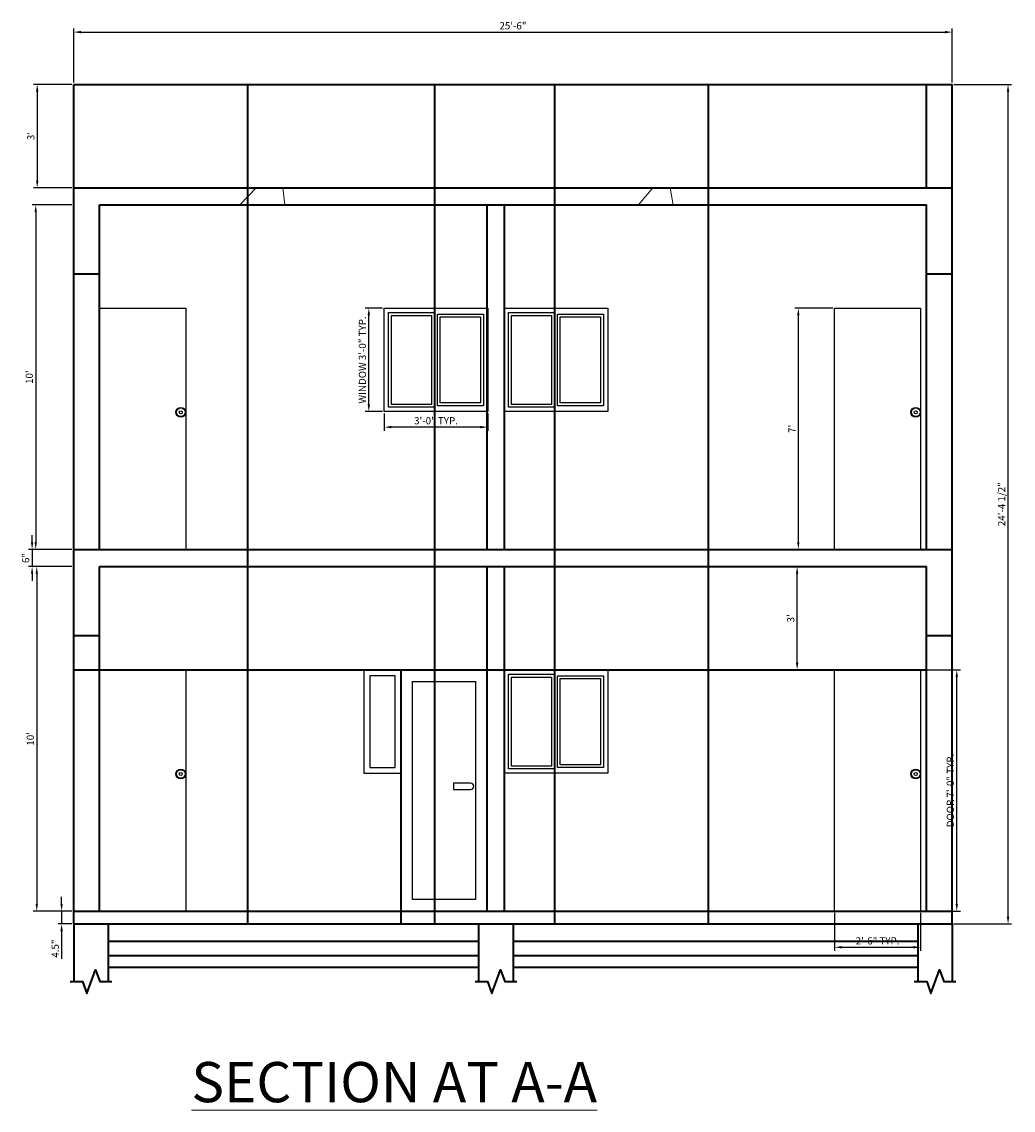
# Model space of a CAD drawing. Units: inches. Extents: x 2117 to 3047, y 1240 to 2266.
# Tile 4 of 4: x 2609 to 2954, y 1884 to 2264. Entities that reach past the tile are written whole.
import ezdxf

# ---------------------------------------------------------------- set-up
doc = ezdxf.new("R2010")
doc.units = ezdxf.units.IN
for name, color, linetype, lineweight in [('A-ANNO-DIMS', 2, 'Continuous', 18), ('A-ANNO-TEXT', 7, 'Continuous', 18), ('A-DOOR', 3, 'Continuous', 25), ('A-GLAZ', 4, 'Continuous', 25), ('A-SECT', 7, 'Continuous', 35), ('A-SECT-PATT', 8, 'Continuous', 13)]:
    doc.layers.add(name, color=color, linetype=linetype, lineweight=lineweight)
doc.styles.get("Standard").update_dxf_attribs({"font": 'arial.ttf'})
doc.dimstyles.new('ISO-25', dxfattribs={"dimtxt": 2.5, "dimasz": 2.5, "dimexe": 1.25, "dimexo": 0.625, "dimtad": 1, "dimdec": 1, "dimlunit": 3, "dimtxsty": 'Standard', "dimcen": 2.5, "dimadec": 0, "dimazin": 0, "dimtfac": 1, "dimtdec": 1, "dimtmove": 0, "dimatfit": 3, "dimfxl": 1, "dimarcsym": 0})

# ---------------------------------------------------------------- blocks, each defined once
blk = doc.blocks.new('Window - Wood Frame 36 x 36 in.')
for p, q in [((2.5, 19.5), (33.5, 19.5)), ((1.5, 18.5), (34.5, 18.5)), ((2, 17.5), (34, 17.5)), ((3, 16.5), (33, 16.5))]:
    blk.add_line(p, q)
blk.add_lwpolyline([(0, 0), (0, 36), (36, 36), (36, 0)], close=True)
for points in [[(1.5, 18.5), (1.5, 34.5), (34.5, 34.5), (34.5, 18.5)], [(2.5, 19.5), (2.5, 33.5), (33.5, 33.5), (33.5, 19.5)], [(34, 17.5), (34, 1.5), (2, 1.5), (2, 17.5)], [(33, 16.5), (33, 2.5), (3, 2.5), (3, 16.5)]]:
    blk.add_lwpolyline(points)
blk = doc.blocks.new('*D7')
at = {"layer": 'A-ANNO-DIMS', "color": 0, "lineweight": -2, "transparency": 16777216}
for p, q in [((2626.24, 2241.7), (2612.89, 2241.7)), ((2614.14, 2239.2), (2614.14, 2208.2)), ((2626.24, 2205.7), (2612.89, 2205.7))]:
    blk.add_line(p, q, dxfattribs=at)
at = {"layer": 'A-ANNO-DIMS', "color": 0, "transparency": 16777216}
for points in [[(2613.72, 2239.2), (2614.55, 2239.2), (2614.14, 2241.7)], [(2613.72, 2208.2), (2614.55, 2208.2), (2614.14, 2205.7)]]:
    blk.add_solid(points, dxfattribs=at)
at = {"layer": 'Defpoints', "color": 0, "transparency": 16777216}
for p in [(2626.86, 2241.7), (2614.14, 2205.7), (2626.86, 2205.7)]:
    blk.add_point(p, dxfattribs=at)
at = {"layer": 'A-ANNO-DIMS', "color": 0, "transparency": 16777216, "insert": (2612.23, 2223.7), "char_height": 2.5, "attachment_point": 5, "rotation": 90}
blk.add_mtext("3'", dxfattribs=at)
blk = doc.blocks.new('*D8')
at = {"layer": 'A-ANNO-DIMS', "color": 0, "lineweight": -2, "transparency": 16777216}
for p, q in [((2626.24, 2199.7), (2612.37, 2199.7)), ((2613.62, 2197.2), (2613.62, 2082.2)), ((2626.24, 2079.7), (2612.37, 2079.7))]:
    blk.add_line(p, q, dxfattribs=at)
at = {"layer": 'A-ANNO-DIMS', "color": 0, "transparency": 16777216}
for points in [[(2613.2, 2197.2), (2614.03, 2197.2), (2613.62, 2199.7)], [(2613.2, 2082.2), (2614.03, 2082.2), (2613.62, 2079.7)]]:
    blk.add_solid(points, dxfattribs=at)
at = {"layer": 'Defpoints', "color": 0, "transparency": 16777216}
for p in [(2626.86, 2199.7), (2613.62, 2079.7), (2626.86, 2079.7)]:
    blk.add_point(p, dxfattribs=at)
at = {"layer": 'A-ANNO-DIMS', "color": 0, "transparency": 16777216, "insert": (2611.71, 2139.7), "char_height": 2.5, "attachment_point": 5, "rotation": 90}
blk.add_mtext("10'", dxfattribs=at)
blk = doc.blocks.new('*D9')
at = {"layer": 'A-ANNO-DIMS', "color": 0, "lineweight": -2, "transparency": 16777216}
for p, q in [((2612.37, 2082.2), (2612.37, 2084.7)), ((2626.24, 2079.7), (2611.12, 2079.7)), ((2612.37, 2079.7), (2612.37, 2073.7)), ((2626.24, 2073.7), (2611.12, 2073.7)), ((2612.37, 2071.2), (2612.37, 2068.7))]:
    blk.add_line(p, q, dxfattribs=at)
at = {"layer": 'A-ANNO-DIMS', "color": 0, "transparency": 16777216}
for points in [[(2611.95, 2082.2), (2612.78, 2082.2), (2612.37, 2079.7)], [(2611.95, 2071.2), (2612.78, 2071.2), (2612.37, 2073.7)]]:
    blk.add_solid(points, dxfattribs=at)
at = {"layer": 'Defpoints', "color": 0, "transparency": 16777216}
for p in [(2626.86, 2079.7), (2612.37, 2073.7), (2626.86, 2073.7)]:
    blk.add_point(p, dxfattribs=at)
at = {"layer": 'A-ANNO-DIMS', "color": 0, "transparency": 16777216, "insert": (2610.46, 2076.7), "char_height": 2.5, "attachment_point": 5, "rotation": 90}
blk.add_mtext('6"', dxfattribs=at)
blk = doc.blocks.new('*D10')
at = {"layer": 'A-ANNO-DIMS', "color": 0, "lineweight": -2, "transparency": 16777216}
for p, q in [((2626.24, 2073.7), (2612.73, 2073.7)), ((2613.98, 2071.2), (2613.98, 1956.2)), ((2626.24, 1953.7), (2612.73, 1953.7))]:
    blk.add_line(p, q, dxfattribs=at)
at = {"layer": 'A-ANNO-DIMS', "color": 0, "transparency": 16777216}
for points in [[(2613.57, 2071.2), (2614.4, 2071.2), (2613.98, 2073.7)], [(2613.57, 1956.2), (2614.4, 1956.2), (2613.98, 1953.7)]]:
    blk.add_solid(points, dxfattribs=at)
at = {"layer": 'Defpoints', "color": 0, "transparency": 16777216}
for p in [(2626.86, 2073.7), (2613.98, 1953.7), (2626.86, 1953.7)]:
    blk.add_point(p, dxfattribs=at)
at = {"layer": 'A-ANNO-DIMS', "color": 0, "transparency": 16777216, "insert": (2612.08, 2013.7), "char_height": 2.5, "attachment_point": 5, "rotation": 90}
blk.add_mtext("10'", dxfattribs=at)
blk = doc.blocks.new('*D11')
at = {"layer": 'A-ANNO-DIMS', "color": 0, "lineweight": -2, "transparency": 16777216}
for p, q in [((2622.64, 1956.2), (2622.64, 1958.7)), ((2626.24, 1953.7), (2621.39, 1953.7)), ((2622.64, 1953.7), (2622.64, 1949.2)), ((2626.24, 1949.2), (2621.39, 1949.2)), ((2622.64, 1946.7), (2622.64, 1937.06))]:
    blk.add_line(p, q, dxfattribs=at)
at = {"layer": 'A-ANNO-DIMS', "color": 0, "transparency": 16777216}
for points in [[(2622.23, 1956.2), (2623.06, 1956.2), (2622.64, 1953.7)], [(2622.23, 1946.7), (2623.06, 1946.7), (2622.64, 1949.2)]]:
    blk.add_solid(points, dxfattribs=at)
at = {"layer": 'Defpoints', "color": 0, "transparency": 16777216}
for p in [(2626.86, 1953.7), (2622.64, 1949.2), (2626.86, 1949.2)]:
    blk.add_point(p, dxfattribs=at)
at = {"layer": 'A-ANNO-DIMS', "color": 0, "transparency": 16777216, "insert": (2620.75, 1940.63), "char_height": 2.5, "attachment_point": 5, "rotation": 90}
blk.add_mtext('4.5"', dxfattribs=at)
blk = doc.blocks.new('*D12')
at = {"layer": 'A-ANNO-DIMS', "color": 0, "lineweight": -2, "transparency": 16777216}
for p, q in [((2891.24, 2163.7), (2878.01, 2163.7)), ((2879.26, 2161.2), (2879.26, 2082.2)), ((2879.89, 2079.7), (2880.51, 2079.7))]:
    blk.add_line(p, q, dxfattribs=at)
at = {"layer": 'A-ANNO-DIMS', "color": 0, "transparency": 16777216}
for points in [[(2878.85, 2161.2), (2879.68, 2161.2), (2879.26, 2163.7)], [(2878.85, 2082.2), (2879.68, 2082.2), (2879.26, 2079.7)]]:
    blk.add_solid(points, dxfattribs=at)
at = {"layer": 'Defpoints', "color": 0, "transparency": 16777216}
for p in [(2891.86, 2163.7), (2879.26, 2079.7), (2879.26, 2079.7)]:
    blk.add_point(p, dxfattribs=at)
at = {"layer": 'A-ANNO-DIMS', "color": 0, "transparency": 16777216, "insert": (2877.39, 2121.7), "char_height": 2.5, "attachment_point": 5, "rotation": 90}
blk.add_mtext("7'", dxfattribs=at)
blk = doc.blocks.new('*D13')
at = {"layer": 'A-ANNO-DIMS', "color": 0, "lineweight": -2, "transparency": 16777216}
for p, q in [((2891.24, 2073.7), (2877.6, 2073.7)), ((2878.85, 2040.2), (2878.85, 2071.2)), ((2891.24, 2037.7), (2877.6, 2037.7))]:
    blk.add_line(p, q, dxfattribs=at)
at = {"layer": 'A-ANNO-DIMS', "color": 0, "transparency": 16777216}
for points in [[(2878.43, 2071.2), (2879.26, 2071.2), (2878.85, 2073.7)], [(2878.43, 2040.2), (2879.26, 2040.2), (2878.85, 2037.7)]]:
    blk.add_solid(points, dxfattribs=at)
at = {"layer": 'Defpoints', "color": 0, "transparency": 16777216}
for p in [(2878.85, 2073.7), (2891.86, 2073.7), (2891.86, 2037.7)]:
    blk.add_point(p, dxfattribs=at)
at = {"layer": 'A-ANNO-DIMS', "color": 0, "transparency": 16777216, "insert": (2876.94, 2055.7), "char_height": 2.5, "attachment_point": 5, "rotation": 90}
blk.add_mtext("3'", dxfattribs=at)
blk = doc.blocks.new('DOOR-ELEV-30')
blk.add_lwpolyline([(0, 84), (30, 84), (30, 0), (0, 0)], close=True)
for radius in [1.7, 1.5, 0.524]:
    blk.add_circle((28.3, 47.76), radius)
blk = doc.blocks.new('*D30')
at = {"layer": 'A-ANNO-DIMS', "color": 0, "lineweight": -2, "transparency": 16777216}
for p, q in [((2922.49, 2037.7), (2935.71, 2037.7)), ((2934.46, 1956.2), (2934.46, 2035.2)), ((2922.49, 1953.7), (2935.71, 1953.7))]:
    blk.add_line(p, q, dxfattribs=at)
at = {"layer": 'A-ANNO-DIMS', "color": 0, "transparency": 16777216}
for points in [[(2934.05, 2035.2), (2934.88, 2035.2), (2934.46, 2037.7)], [(2934.05, 1956.2), (2934.88, 1956.2), (2934.46, 1953.7)]]:
    blk.add_solid(points, dxfattribs=at)
at = {"layer": 'Defpoints', "color": 0, "transparency": 16777216}
for p in [(2921.86, 2037.7), (2934.46, 2037.7), (2921.86, 1953.7)]:
    blk.add_point(p, dxfattribs=at)
at = {"layer": 'A-ANNO-DIMS', "color": 0, "transparency": 16777216, "insert": (2932.54, 1995.7), "char_height": 2.5, "attachment_point": 5, "rotation": 90}
blk.add_mtext('DOOR 7\'-0" TYP.', dxfattribs=at)
blk = doc.blocks.new('*D31')
at = {"layer": 'A-ANNO-DIMS', "color": 0, "lineweight": -2, "transparency": 16777216}
for p, q in [((2891.86, 1953.08), (2891.86, 1939.85)), ((2921.86, 1953.08), (2921.86, 1939.85)), ((2894.36, 1941.1), (2919.36, 1941.1))]:
    blk.add_line(p, q, dxfattribs=at)
at = {"layer": 'A-ANNO-DIMS', "color": 0, "transparency": 16777216}
for points in [[(2894.36, 1941.52), (2894.36, 1940.68), (2891.86, 1941.1)], [(2919.36, 1941.52), (2919.36, 1940.68), (2921.86, 1941.1)]]:
    blk.add_solid(points, dxfattribs=at)
at = {"layer": 'Defpoints', "color": 0, "transparency": 16777216}
for p in [(2891.86, 1953.7), (2921.86, 1953.7), (2921.86, 1941.1)]:
    blk.add_point(p, dxfattribs=at)
at = {"layer": 'A-ANNO-DIMS', "color": 0, "transparency": 16777216, "insert": (2906.86, 1943), "char_height": 2.5, "attachment_point": 5}
blk.add_mtext('2\'-6" TYP.', dxfattribs=at)
blk = doc.blocks.new('*D32')
at = {"layer": 'A-ANNO-DIMS', "color": 0, "lineweight": -2, "transparency": 16777216}
for p, q in [((2734.42, 2163.7), (2728.4, 2163.7)), ((2729.65, 2130.2), (2729.65, 2161.2)), ((2734.42, 2127.7), (2728.4, 2127.7))]:
    blk.add_line(p, q, dxfattribs=at)
at = {"layer": 'A-ANNO-DIMS', "color": 0, "transparency": 16777216}
for points in [[(2729.23, 2161.2), (2730.06, 2161.2), (2729.65, 2163.7)], [(2729.23, 2130.2), (2730.06, 2130.2), (2729.65, 2127.7)]]:
    blk.add_solid(points, dxfattribs=at)
at = {"layer": 'Defpoints', "color": 0, "transparency": 16777216}
for p in [(2729.65, 2163.7), (2735.05, 2163.7), (2735.05, 2127.7)]:
    blk.add_point(p, dxfattribs=at)
at = {"layer": 'A-ANNO-DIMS', "color": 0, "transparency": 16777216, "insert": (2727.73, 2145.7), "char_height": 2.5, "attachment_point": 5, "rotation": 90}
blk.add_mtext('WINDOW 3\'-0" TYP.', dxfattribs=at)
blk = doc.blocks.new('*D33')
at = {"layer": 'A-ANNO-DIMS', "color": 0, "lineweight": -2, "transparency": 16777216}
for p, q in [((2735.05, 2127.08), (2735.05, 2121.05)), ((2771.05, 2127.08), (2771.05, 2121.05)), ((2768.55, 2122.3), (2737.55, 2122.3))]:
    blk.add_line(p, q, dxfattribs=at)
at = {"layer": 'A-ANNO-DIMS', "color": 0, "transparency": 16777216}
for points in [[(2737.55, 2122.72), (2737.55, 2121.88), (2735.05, 2122.3)], [(2768.55, 2122.72), (2768.55, 2121.88), (2771.05, 2122.3)]]:
    blk.add_solid(points, dxfattribs=at)
at = {"layer": 'Defpoints', "color": 0, "transparency": 16777216}
for p in [(2735.05, 2127.7), (2771.05, 2127.7), (2735.05, 2122.3)]:
    blk.add_point(p, dxfattribs=at)
at = {"layer": 'A-ANNO-DIMS', "color": 0, "transparency": 16777216, "insert": (2753.05, 2124.2), "char_height": 2.5, "attachment_point": 5}
blk.add_mtext('3\'-0" TYP.', dxfattribs=at)
blk = doc.blocks.new('*D54')
at = {"layer": 'A-ANNO-DIMS', "color": 0, "lineweight": -2, "transparency": 16777216}
for p, q in [((2626.86, 2242.33), (2626.86, 2261.15)), ((2932.86, 2242.33), (2932.86, 2261.15)), ((2629.36, 2259.9), (2930.36, 2259.9))]:
    blk.add_line(p, q, dxfattribs=at)
at = {"layer": 'A-ANNO-DIMS', "color": 0, "transparency": 16777216}
for points in [[(2629.36, 2260.32), (2629.36, 2259.48), (2626.86, 2259.9)], [(2930.36, 2260.32), (2930.36, 2259.48), (2932.86, 2259.9)]]:
    blk.add_solid(points, dxfattribs=at)
at = {"layer": 'Defpoints', "color": 0, "transparency": 16777216}
for p in [(2932.86, 2259.9), (2626.86, 2241.7), (2932.86, 2241.7)]:
    blk.add_point(p, dxfattribs=at)
at = {"layer": 'A-ANNO-DIMS', "color": 0, "transparency": 16777216, "insert": (2779.86, 2261.8), "char_height": 2.5, "attachment_point": 5}
blk.add_mtext('25\'-6"', dxfattribs=at)
blk = doc.blocks.new('*D55')
at = {"layer": 'A-ANNO-DIMS', "color": 0, "lineweight": -2, "transparency": 16777216}
for p, q in [((2933.49, 2241.7), (2953.56, 2241.7)), ((2952.31, 1951.7), (2952.31, 2239.2)), ((2933.49, 1949.2), (2953.56, 1949.2))]:
    blk.add_line(p, q, dxfattribs=at)
at = {"layer": 'A-ANNO-DIMS', "color": 0, "transparency": 16777216}
for points in [[(2951.9, 2239.2), (2952.73, 2239.2), (2952.31, 2241.7)], [(2951.9, 1951.7), (2952.73, 1951.7), (2952.31, 1949.2)]]:
    blk.add_solid(points, dxfattribs=at)
at = {"layer": 'Defpoints', "color": 0, "transparency": 16777216}
for p in [(2932.86, 2241.7), (2952.31, 2241.7), (2932.86, 1949.2)]:
    blk.add_point(p, dxfattribs=at)
at = {"layer": 'A-ANNO-DIMS', "color": 0, "transparency": 16777216, "insert": (2950.39, 2095.45), "char_height": 2.5, "attachment_point": 5, "rotation": 90}
blk.add_mtext('24\'-4 1/2"', dxfattribs=at)

msp = doc.modelspace()

# ---------------------------------------------------------------- hatches: boundary and pattern name
at = {"layer": 'A-SECT-PATT'}
h = msp.add_hatch(dxfattribs=at)
h.set_pattern_fill('AR-CONC', color=256, scale=30)
h.paths.add_polyline_path([(2635.86, 2199.7), (2923.86, 2199.7), (2923.86, 2175.7), (2932.86, 2175.7), (2932.86, 2205.7), (2626.86, 2205.7), (2626.86, 2175.7), (2635.86, 2175.7)])
h.paths.add_polyline_path([(2932.86, 2079.7), (2626.86, 2079.7), (2626.86, 2049.7), (2635.86, 2049.7), (2635.86, 2073.7), (2923.86, 2073.7), (2923.86, 2049.7), (2932.86, 2049.7)])
h = msp.add_hatch(dxfattribs=at)
h.set_pattern_fill('AR-CONC', color=256)
h.paths.add_polyline_path([(2923.86, 2205.7), (2635.86, 2205.7), (2635.86, 2199.7), (2923.86, 2199.7)])
h.paths.add_polyline_path([(2770.86, 2079.7), (2635.86, 2079.7), (2635.86, 2073.7), (2770.86, 2073.7)])
h.paths.add_polyline_path([(2923.86, 2079.7), (2776.86, 2079.7), (2776.86, 2073.7), (2923.86, 2073.7)])
h.paths.add_polyline_path([(2776.86, 2079.7), (2770.86, 2079.7), (2770.86, 2073.7), (2776.86, 2073.7)])
h = msp.add_hatch(dxfattribs=at)
h.set_pattern_fill('AR-CONC', color=256, scale=30)
h.paths.add_polyline_path([(2932.86, 1953.7), (2626.86, 1953.7), (2626.86, 1949.2), (2932.86, 1949.2)])

# ---------------------------------------------------------------- linework, layer by layer
at = {"layer": 'A-DOOR'}
for points in [[(2740.86, 2037.7), (2770.86, 2037.7), (2770.86, 1953.7), (2740.86, 1953.7)], [(2744.86, 2033.7), (2766.86, 2033.7), (2766.86, 1957.7), (2744.86, 1957.7)]]:
    msp.add_lwpolyline(points, close=True, dxfattribs=at)
msp.add_lwpolyline([(2765.11, 1998.27), (2759.2, 1998.27), (2759.2, 1996.06), (2765.11, 1996.06), (2765.11, 1996.07)], dxfattribs=at)
msp.add_arc((2765.11, 1997.17), 1.1, 270, 90, dxfattribs=at)
at = {"layer": 'A-GLAZ'}
for points in [[(2740.86, 2037.7), (2727.97, 2037.7), (2727.97, 2001.7), (2740.86, 2001.7)], [(2738.86, 2035.7), (2729.97, 2035.7), (2729.97, 2003.7), (2738.86, 2003.7)]]:
    msp.add_lwpolyline(points, close=True, dxfattribs=at)
at = {"layer": 'A-SECT'}
for p, q in [((2626.86, 1949.2), (2626.86, 2241.7)), ((2626.86, 2241.7), (2932.86, 2241.7)), ((2687.36, 2241.7), (2687.36, 1949.2)), ((2752.55, 2241.7), (2752.55, 1949.2)), ((2794.36, 2241.7), (2794.36, 1949.2)), ((2847.86, 2241.7), (2847.86, 1949.2)), ((2923.86, 2205.7), (2923.86, 2241.7)), ((2932.86, 1949.2), (2932.86, 2241.7)), ((2626.86, 2205.7), (2932.86, 2205.7)), ((2635.86, 2199.7), (2923.86, 2199.7)), ((2635.86, 2079.7), (2635.86, 2199.7)), ((2770.86, 2079.7), (2770.86, 2199.7)), ((2776.86, 2079.7), (2776.86, 2199.7)), ((2923.86, 2079.7), (2923.86, 2199.7)), ((2626.86, 2175.7), (2635.86, 2175.7)), ((2923.86, 2175.7), (2932.86, 2175.7)), ((2626.86, 2079.7), (2932.86, 2079.7)), ((2635.86, 1953.7), (2635.86, 2073.7)), ((2635.86, 2073.7), (2923.86, 2073.7)), ((2770.86, 1953.7), (2770.86, 2073.7)), ((2776.86, 1953.7), (2776.86, 2073.7)), ((2923.86, 1953.7), (2923.86, 2073.7)), ((2626.86, 2049.7), (2635.86, 2049.7)), ((2923.86, 2049.7), (2932.86, 2049.7)), ((2626.86, 2037.7), (2923.86, 2037.7)), ((2740.86, 2037.7), (2740.86, 1949.2)), ((2626.86, 1953.7), (2932.86, 1953.7)), ((2626.86, 1949.2), (2932.86, 1949.2)), ((2626.86, 1949.2), (2626.86, 1929.16)), ((2638.86, 1949.2), (2638.86, 1929.16)), ((2767.91, 1949.2), (2767.91, 1929.16)), ((2779.91, 1949.2), (2779.91, 1929.16)), ((2920.86, 1949.2), (2920.86, 1929.16)), ((2932.86, 1949.2), (2932.86, 1929.16)), ((2638.86, 1943.2), (2767.91, 1943.2)), ((2779.91, 1943.2), (2920.86, 1943.2)), ((2638.86, 1938.2), (2767.91, 1938.2)), ((2779.91, 1938.2), (2920.86, 1938.2)), ((2638.86, 1934.2), (2767.91, 1934.2)), ((2779.91, 1934.2), (2920.86, 1934.2))]:
    msp.add_line(p, q, dxfattribs=at)
for points in [[(2625.61, 1929.16), (2629.97, 1929.16), (2631.47, 1925.04), (2634.47, 1933.28), (2635.97, 1929.16), (2640.11, 1929.16)], [(2766.66, 1929.16), (2771.01, 1929.16), (2772.51, 1925.04), (2775.51, 1933.28), (2777.01, 1929.16), (2781.16, 1929.16)], [(2919.61, 1929.16), (2923.97, 1929.16), (2925.47, 1925.04), (2928.47, 1933.28), (2929.97, 1929.16), (2934.11, 1929.16)]]:
    msp.add_lwpolyline(points, dxfattribs=at)

# ---------------------------------------------------------------- block references
at = {"layer": 'A-DOOR'}
for p in [(2635.86, 2079.7), (2891.86, 2079.7), (2635.86, 1953.7), (2891.86, 1953.7)]:
    msp.add_blockref('DOOR-ELEV-30', p, dxfattribs=at)
at = {"layer": 'A-GLAZ', "rotation": 90}
for p in [(2771.05, 2127.7), (2812.86, 2127.7), (2812.86, 2001.7)]:
    msp.add_blockref('Window - Wood Frame 36 x 36 in.', p, dxfattribs=at)

# ---------------------------------------------------------------- texts
at = {"layer": 'A-ANNO-TEXT', "insert": (2667.84, 1901.12), "char_height": 14, "attachment_point": 1}
msp.add_mtext_dynamic_manual_height_columns('{\\LSECTION AT A-A}', width=221.8965, gutter_width=70, heights=[0], dxfattribs=at)

# ---------------------------------------------------------------- dimensions: what is measured, and where the dimension line sits
at = {"layer": 'A-ANNO-DIMS'}
dim = msp.add_linear_dim(base=(2932.86, 2259.9), p1=(2626.86, 2241.7), p2=(2932.86, 2241.7), dimstyle='ISO-25', override={"dimdec": 1, "dimlfac": 1, "dimrnd": 0, "dimzin": 1, "dimdsep": 46, "dimlunit": 4, "dimfrac": 2}, dxfattribs=at)
dim.commit()
dim.dimension.update_dxf_attribs({"geometry": '*D54', "text_midpoint": (2779.86, 2261.8)})
for base, p1, p2, override, picture, middle in [((2614.14, 2205.7), (2626.86, 2241.7), (2626.86, 2205.7), {"dimclrd": 0, "dimclre": 0, "dimclrt": 0}, '*D7', (2612.23, 2223.7)), ((2952.31, 2241.7), (2932.86, 1949.2), (2932.86, 2241.7), {"dimdec": 1, "dimlfac": 1, "dimrnd": 0, "dimzin": 1, "dimdsep": 46, "dimlunit": 4, "dimfrac": 2}, '*D55', (2950.39, 2095.45)), ((2613.62, 2079.7), (2626.86, 2199.7), (2626.86, 2079.7), {"dimclrd": 0, "dimclre": 0, "dimclrt": 0}, '*D8', (2611.71, 2139.7)), ((2879.26, 2079.7), (2891.86, 2163.7), (2879.26, 2079.7), {"dimclrd": 0, "dimclre": 0, "dimclrt": 0}, '*D12', (2877.39, 2121.7)), ((2612.37, 2073.7), (2626.86, 2079.7), (2626.86, 2073.7), {"dimclrd": 0, "dimclre": 0, "dimclrt": 0}, '*D9', (2610.46, 2076.7)), ((2613.98, 1953.7), (2626.86, 2073.7), (2626.86, 1953.7), {"dimclrd": 0, "dimclre": 0, "dimclrt": 0}, '*D10', (2612.08, 2013.7)), ((2878.85, 2073.7), (2891.86, 2037.7), (2891.86, 2073.7), {"dimclrd": 0, "dimclre": 0, "dimclrt": 0}, '*D13', (2876.94, 2055.7)), ((2622.64, 1949.2), (2626.86, 1953.7), (2626.86, 1949.2), {"dimclrd": 0, "dimclre": 0, "dimclrt": 0}, '*D11', (2620.75, 1940.63))]:
    dim = msp.add_linear_dim(base=base, p1=p1, p2=p2, angle=90, dimstyle='ISO-25', override=override, dxfattribs=at)
    dim.commit()
    dim.dimension.update_dxf_attribs({"geometry": picture, "text_midpoint": middle})
for base, p1, p2, angle, text, picture, middle in [((2729.65, 2163.7), (2735.05, 2127.7), (2735.05, 2163.7), 90, 'WINDOW <> TYP.', '*D32', (2727.73, 2145.7)), ((2735.05, 2122.3), (2771.05, 2127.7), (2735.05, 2127.7), 180, '<> TYP.', '*D33', (2753.05, 2124.2)), ((2934.46, 2037.7), (2921.86, 1953.7), (2921.86, 2037.7), 90, 'DOOR <> TYP.', '*D30', (2932.54, 1995.7))]:
    dim = msp.add_linear_dim(base=base, p1=p1, p2=p2, angle=angle, text=text, dimstyle='ISO-25', override={"dimdec": 1, "dimrnd": 0, "dimzin": 1, "dimlunit": 4, "dimfrac": 2}, dxfattribs=at)
    dim.commit()
    dim.dimension.update_dxf_attribs({"geometry": picture, "text_midpoint": middle})
dim = msp.add_linear_dim(base=(2921.86, 1941.1), p1=(2891.86, 1953.7), p2=(2921.86, 1953.7), text='<> TYP.', dimstyle='ISO-25', override={"dimdec": 1, "dimrnd": 0, "dimzin": 1, "dimlunit": 4, "dimfrac": 2}, dxfattribs=at)
dim.commit()
dim.dimension.update_dxf_attribs({"geometry": '*D31', "text_midpoint": (2906.86, 1943)})

doc.saveas('drawing.dxf')
